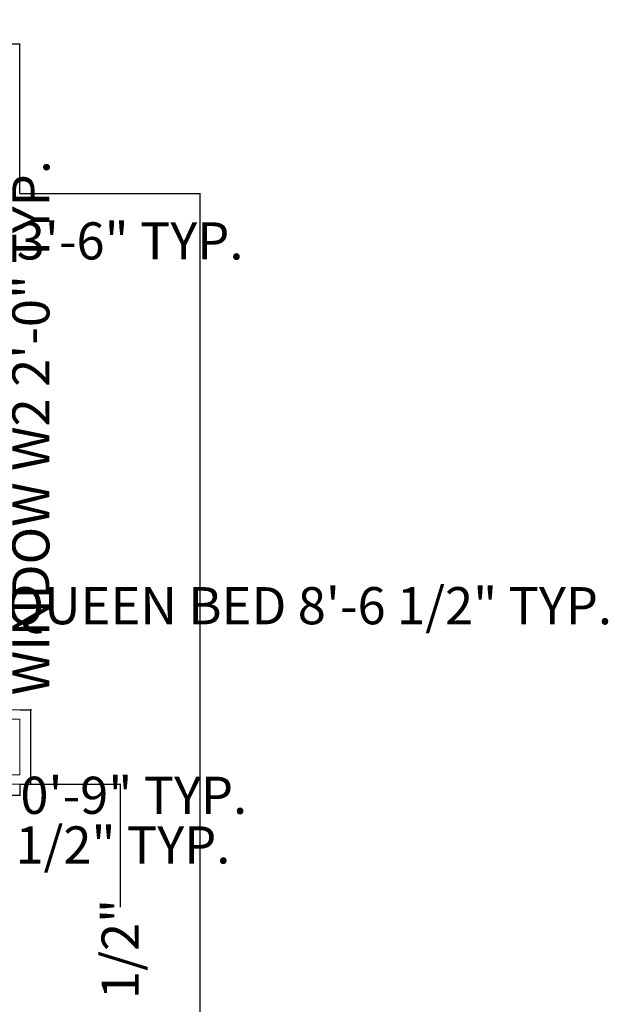
# Model space of a CAD drawing. Units: inches. Extents: x -51 to 1118, y -44 to 791.
# Tile 7 of 8: x 340 to 530, y 344 to 662. Entities that reach past the tile are written whole.
import ezdxf

# ---------------------------------------------------------------- set-up
doc = ezdxf.new("R2010")
doc.units = ezdxf.units.IN
doc.header["$MEASUREMENT"] = 0
doc.layers.add('A-ANNO-DIMS', color=2, linetype='Continuous', lineweight=18)
doc.layers.add('A-GLAZ', color=4, linetype='Continuous', lineweight=18)
doc.styles.get("Standard").update_dxf_attribs({"font": 'arial.ttf'})
doc.dimstyles.get("Standard").update_dxf_attribs({"dimtxt": 12, "dimasz": 0.18, "dimexe": 0.18, "dimexo": 0.0625, "dimgap": 0.09, "dimtad": 0, "dimdec": 1, "dimzin": 0, "dimdsep": 46, "dimlunit": 3, "dimtxsty": 'Standard', "dimcen": 0.09, "dimadec": 0, "dimazin": 0, "dimtfac": 1, "dimtdec": 1, "dimtofl": 0, "dimtmove": 0, "dimatfit": 3, "dimfxl": 1, "dimtolj": 1, "dimtzin": 0, "dimarcsym": 0})

# ---------------------------------------------------------------- blocks, each defined once
blk = doc.blocks.new('*D9')
at = {"layer": 'A-ANNO-DIMS', "color": 0, "lineweight": -2, "transparency": 16777216}
for p, q in [((340.08, 605.94), (398.42, 605.94)), ((398.24, 605.76), (398.24, 316.21)), ((398.24, 6.12), (398.24, 295.67)), ((340.08, 5.94), (398.42, 5.94))]:
    blk.add_line(p, q, dxfattribs=at)
at = {"layer": 'A-ANNO-DIMS', "color": 0, "transparency": 16777216}
for points in [[(398.21, 605.76), (398.27, 605.76), (398.24, 605.94)], [(398.21, 6.12), (398.27, 6.12), (398.24, 5.94)]]:
    blk.add_solid(points, dxfattribs=at)
at = {"layer": 'Defpoints', "color": 0, "transparency": 16777216}
for p in [(340.02, 605.94), (340.02, 5.94), (398.24, 5.94)]:
    blk.add_point(p, dxfattribs=at)
at = {"layer": 'A-ANNO-DIMS', "color": 0, "transparency": 16777216, "insert": (398.24, 305.94), "char_height": 12, "attachment_point": 5, "rotation": 90}
blk.add_mtext("\\A1;50'", dxfattribs=at)
blk = doc.blocks.new('*D10')
at = {"layer": 'A-ANNO-DIMS', "color": 0, "lineweight": -2, "transparency": 16777216}
for p, q in [((28.02, 606), (28.02, 654.38)), ((28.2, 654.2), (173.65, 654.2)), ((339.84, 654.2), (194.4, 654.2)), ((340.02, 606), (340.02, 654.38))]:
    blk.add_line(p, q, dxfattribs=at)
at = {"layer": 'A-ANNO-DIMS', "color": 0, "transparency": 16777216}
for points in [[(28.2, 654.23), (28.2, 654.17), (28.02, 654.2)], [(339.84, 654.23), (339.84, 654.17), (340.02, 654.2)]]:
    blk.add_solid(points, dxfattribs=at)
at = {"layer": 'Defpoints', "color": 0, "transparency": 16777216}
for p in [(340.02, 654.2), (28.02, 605.94), (340.02, 605.94)]:
    blk.add_point(p, dxfattribs=at)
at = {"layer": 'A-ANNO-DIMS', "color": 0, "transparency": 16777216, "insert": (184.02, 654.2), "char_height": 12, "attachment_point": 5}
blk.add_mtext("\\A1;26'", dxfattribs=at)
blk = doc.blocks.new('WIN-18IN')
for p, q in [((9, 24), (0, 24)), ((0, 21), (0, 3)), ((9, 21), (0, 21)), ((1.5, 21), (1.5, 3)), ((4.5, 21), (4.5, 3)), ((9, 3), (9, 21)), ((0, 3), (9, 3)), ((0, 0), (9, 0))]:
    blk.add_line(p, q)
blk = doc.blocks.new('*D16')
at = {"layer": 'A-ANNO-DIMS', "color": 0, "lineweight": -2, "transparency": 16777216}
for p, q in [((192.77, 596.88), (192.77, 590.46)), ((234.77, 596.88), (234.77, 590.46)), ((192.95, 590.64), (234.59, 590.64)), ((234.77, 590.64), (234.95, 590.64))]:
    blk.add_line(p, q, dxfattribs=at)
at = {"layer": 'A-ANNO-DIMS', "color": 0, "transparency": 16777216}
for points in [[(192.95, 590.67), (192.95, 590.61), (192.77, 590.64)], [(234.59, 590.67), (234.59, 590.61), (234.77, 590.64)]]:
    blk.add_solid(points, dxfattribs=at)
at = {"layer": 'Defpoints', "color": 0, "transparency": 16777216}
for p in [(192.77, 596.94), (234.77, 596.94), (234.77, 590.64)]:
    blk.add_point(p, dxfattribs=at)
at = {"layer": 'A-ANNO-DIMS', "color": 0, "transparency": 16777216, "insert": (325.87, 590.64), "char_height": 12, "attachment_point": 5}
blk.add_mtext('\\A1;WINDOW W1 3\'-6" TYP.', dxfattribs=at)
blk = doc.blocks.new('*D18')
at = {"layer": 'A-ANNO-DIMS', "color": 0, "lineweight": -2, "transparency": 16777216}
for p, q in [((340.08, 439.22), (343.8, 439.22)), ((343.62, 439.22), (343.62, 439.4)), ((343.62, 415.4), (343.62, 439.04)), ((340.08, 415.22), (343.8, 415.22))]:
    blk.add_line(p, q, dxfattribs=at)
at = {"layer": 'A-ANNO-DIMS', "color": 0, "transparency": 16777216}
for points in [[(343.59, 439.04), (343.65, 439.04), (343.62, 439.22)], [(343.59, 415.4), (343.65, 415.4), (343.62, 415.22)]]:
    blk.add_solid(points, dxfattribs=at)
at = {"layer": 'Defpoints', "color": 0, "transparency": 16777216}
for p in [(340.02, 439.22), (343.62, 439.22), (340.02, 415.22)]:
    blk.add_point(p, dxfattribs=at)
at = {"layer": 'A-ANNO-DIMS', "color": 0, "transparency": 16777216, "insert": (343.62, 530.31), "char_height": 12, "attachment_point": 5, "rotation": 90}
blk.add_mtext('\\A1;WINDOW W2 2\'-0" TYP.', dxfattribs=at)
blk = doc.blocks.new('*D19')
at = {"layer": 'A-ANNO-DIMS', "color": 0, "lineweight": -2, "transparency": 16777216}
for p, q in [((331.02, 415.15), (331.02, 411.44)), ((340.02, 415.15), (340.02, 411.44)), ((331.2, 411.62), (339.84, 411.62)), ((340.02, 411.62), (340.2, 411.62))]:
    blk.add_line(p, q, dxfattribs=at)
at = {"layer": 'A-ANNO-DIMS', "color": 0, "transparency": 16777216}
for points in [[(331.2, 411.65), (331.2, 411.59), (331.02, 411.62)], [(339.84, 411.65), (339.84, 411.59), (340.02, 411.62)]]:
    blk.add_solid(points, dxfattribs=at)
at = {"layer": 'Defpoints', "color": 0, "transparency": 16777216}
for p in [(331.02, 415.22), (340.02, 415.22), (340.02, 411.62)]:
    blk.add_point(p, dxfattribs=at)
at = {"layer": 'A-ANNO-DIMS', "color": 0, "transparency": 16777216, "insert": (376.86, 411.62), "char_height": 12, "attachment_point": 5}
blk.add_mtext('\\A1;0\'-9" TYP.', dxfattribs=at)
blk = doc.blocks.new('*D22')
at = {"layer": 'A-ANNO-DIMS', "color": 0, "lineweight": -2, "transparency": 16777216}
for p, q in [((187.02, 401.88), (187.02, 395.4)), ((229.44, 401.88), (229.44, 395.4)), ((187.2, 395.58), (229.26, 395.58)), ((229.44, 395.58), (229.62, 395.58))]:
    blk.add_line(p, q, dxfattribs=at)
at = {"layer": 'A-ANNO-DIMS', "color": 0, "transparency": 16777216}
for points in [[(187.2, 395.61), (187.2, 395.55), (187.02, 395.58)], [(229.26, 395.61), (229.26, 395.55), (229.44, 395.58)]]:
    blk.add_solid(points, dxfattribs=at)
at = {"layer": 'Defpoints', "color": 0, "transparency": 16777216}
for p in [(187.02, 401.94), (229.44, 401.94), (229.44, 395.58)]:
    blk.add_point(p, dxfattribs=at)
at = {"layer": 'A-ANNO-DIMS', "color": 0, "transparency": 16777216, "insert": (320.49, 395.58), "char_height": 12, "attachment_point": 5}
blk.add_mtext('\\A1;DOOR D2 3\'-6 1/2" TYP.', dxfattribs=at)
blk = doc.blocks.new('*D26')
at = {"layer": 'A-ANNO-DIMS', "color": 0, "lineweight": -2, "transparency": 16777216}
for p, q in [((228.63, 488.13), (228.63, 472.66)), ((331.02, 488.13), (331.02, 472.66)), ((228.81, 472.84), (330.84, 472.84)), ((331.02, 472.84), (331.2, 472.84))]:
    blk.add_line(p, q, dxfattribs=at)
at = {"layer": 'A-ANNO-DIMS', "color": 0, "transparency": 16777216}
for points in [[(228.81, 472.87), (228.81, 472.81), (228.63, 472.84)], [(330.84, 472.87), (330.84, 472.81), (331.02, 472.84)]]:
    blk.add_solid(points, dxfattribs=at)
at = {"layer": 'Defpoints', "color": 0, "transparency": 16777216}
for p in [(228.63, 488.2), (331.02, 488.2), (331.02, 472.84)]:
    blk.add_point(p, dxfattribs=at)
at = {"layer": 'A-ANNO-DIMS', "color": 0, "transparency": 16777216, "insert": (433.53, 472.84), "char_height": 12, "attachment_point": 5}
blk.add_mtext('\\A1;QUEEN BED 8\'-6 1/2" TYP.', dxfattribs=at)
blk = doc.blocks.new('*D52')
at = {"layer": 'A-ANNO-DIMS', "color": 0, "lineweight": -2, "transparency": 16777216}
for p, q in [((340.08, 415.22), (372.65, 415.22)), ((372.47, 415.04), (372.47, 375.54)), ((372.47, 267.81), (372.47, 307.31)), ((340.08, 267.63), (372.65, 267.63))]:
    blk.add_line(p, q, dxfattribs=at)
at = {"layer": 'A-ANNO-DIMS', "color": 0, "transparency": 16777216}
for points in [[(372.44, 415.04), (372.5, 415.04), (372.47, 415.22)], [(372.44, 267.81), (372.5, 267.81), (372.47, 267.63)]]:
    blk.add_solid(points, dxfattribs=at)
at = {"layer": 'Defpoints', "color": 0, "transparency": 16777216}
for p in [(340.02, 415.22), (372.47, 415.22), (340.02, 267.63)]:
    blk.add_point(p, dxfattribs=at)
at = {"layer": 'A-ANNO-DIMS', "color": 0, "transparency": 16777216, "insert": (372.47, 341.42), "char_height": 12, "attachment_point": 5, "rotation": 90}
blk.add_mtext('\\A1;12\'-3 1/2"', dxfattribs=at)

msp = doc.modelspace()

# ---------------------------------------------------------------- block references
at = {"layer": 'A-GLAZ'}
msp.add_blockref('WIN-18IN', (331.02, 415.22), dxfattribs=at)

# ---------------------------------------------------------------- dimensions: what is measured, and where the dimension line sits
at = {"layer": 'A-ANNO-DIMS'}
dim = msp.add_linear_dim(base=(340.02, 654.2), p1=(28.02, 605.94), p2=(340.02, 605.94), dimstyle='Standard', override={"dimclrd": 0, "dimclre": 0, "dimclrt": 0}, dxfattribs=at)
dim.commit()
dim.dimension.update_dxf_attribs({"geometry": '*D10', "text_midpoint": (184.02, 654.2)})
for base, p1, p2, angle, text, picture, middle in [((234.77, 590.64), (192.77, 596.94), (234.77, 596.94), 0, 'WINDOW W1 <> TYP.', '*D16', (325.87, 590.64)), ((343.62, 439.22), (340.02, 415.22), (340.02, 439.22), 90, 'WINDOW W2 <> TYP.', '*D18', (343.62, 530.31))]:
    dim = msp.add_linear_dim(base=base, p1=p1, p2=p2, angle=angle, text=text, dimstyle='Standard', override={"dimdec": 1, "dimlfac": 1, "dimrnd": 0, "dimzin": 1, "dimdsep": 46, "dimlunit": 4, "dimfrac": 2}, dxfattribs=at)
    dim.commit()
    dim.dimension.update_dxf_attribs({"geometry": picture, "text_midpoint": middle})
for base, p1, p2, override, picture, middle in [((398.24, 5.94), (340.02, 605.94), (340.02, 5.94), {"dimclrd": 0, "dimclre": 0, "dimclrt": 0}, '*D9', (398.24, 305.94)), ((372.47, 415.22), (340.02, 267.63), (340.02, 415.22), {"dimdec": 1, "dimlfac": 1, "dimrnd": 0, "dimzin": 1, "dimdsep": 46, "dimlunit": 4, "dimfrac": 2}, '*D52', (372.47, 341.42))]:
    dim = msp.add_linear_dim(base=base, p1=p1, p2=p2, angle=90, dimstyle='Standard', override=override, dxfattribs=at)
    dim.commit()
    dim.dimension.update_dxf_attribs({"geometry": picture, "text_midpoint": middle})
for base, p1, p2, text, picture, middle in [((331.02, 472.84), (228.63, 488.2), (331.02, 488.2), 'QUEEN BED <> TYP.', '*D26', (433.53, 472.84)), ((229.44, 395.58), (187.02, 401.94), (229.44, 401.94), 'DOOR D2 <> TYP.', '*D22', (320.49, 395.58)), ((340.02, 411.62), (331.02, 415.22), (340.02, 415.22), '<> TYP.', '*D19', (376.86, 411.62))]:
    dim = msp.add_linear_dim(base=base, p1=p1, p2=p2, text=text, dimstyle='Standard', override={"dimdec": 1, "dimlfac": 1, "dimrnd": 0, "dimzin": 1, "dimdsep": 46, "dimlunit": 4, "dimfrac": 2}, dxfattribs=at)
    dim.commit()
    dim.dimension.update_dxf_attribs({"geometry": picture, "text_midpoint": middle})

doc.saveas('drawing.dxf')
